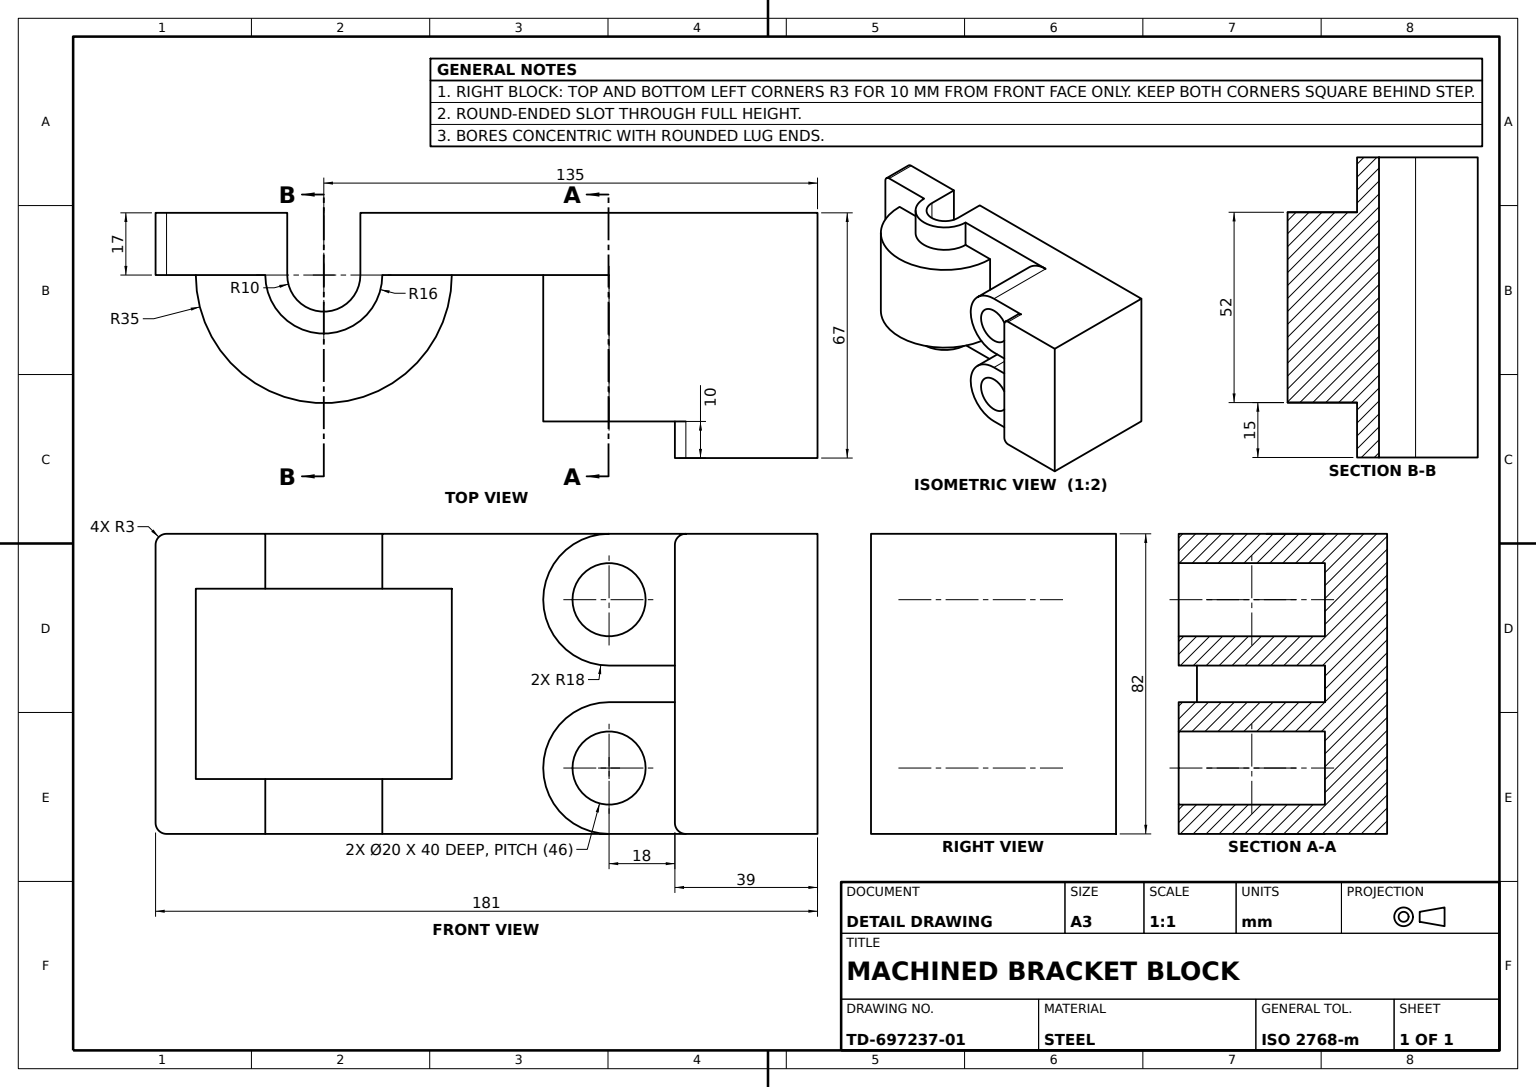
SolidWorks part; units mm, degrees
material "Plain Carbon Steel"
ref_plane "Front Plane" through (0, 0, 0) normal (0, 0, 1) x (1, 0, 0)
ref_plane "Top Plane" through (0, 0, 0) normal (0, 1, 0) x (1, 0, 0)
ref_plane "Right Plane" through (0, 0, 0) normal (1, 0, 0) x (0, 0, -1)
sketch "Base Block Sketch" plane through (0, 0, 0) normal (0, 0, 1) x (1, 0, 0)
  line L3 (0, 0) -> (175, 0)
  line L4 (175, 0) -> (175, 82)
  line L5 (175, 82) -> (0, 82)
  line L6 (0, 82) -> (0, 0)
  dimension "D1" = 175
  dimension "D2" = 82
extrude "Base Block" add sketch "Base Block Sketch" along normal blind 17
sketch "Side Wall Sketch" plane through (0, 0, 17) normal (0, 0, 1) x (1, 0, 0)
  line L0 (175, 82) -> (175, 0)
  line L1 (175, 0) -> (139, 0)
  line L2 (0, 0) -> (175, 0) construction
  line L3 (0, 82) -> (0, 0) construction
  line L4 (175, 82) -> (139, 82)
  line L5 (175, 82) -> (0, 82) construction
  line L7 (136, 79) -> (136, 3)
  arc A0 (136, 3) -> (139, 0) centre (139, 3) ccw
  arc A1 (139, 82) -> (136, 79) centre (139, 79) ccw
  dimension "D1" = 6
  dimension "D2" = 6
  dimension "D3" = 3
  dimension "D4" = 136
extrude "Side Wall" add sketch "Side Wall Sketch" along normal blind 50
sketch "Step Pad Sketch" plane through (0, 0, 0) normal (-1, 0, 0) x (0, 0, 1)
  line L0 (0, 82) -> (17, 82)
  line L1 (17, 82) -> (17, 0)
  line L2 (17, 82) -> (17, 0) construction
  line L3 (17, 0) -> (0, 0) construction
  line L4 (17, 0) -> (0, 0)
  line L5 (0, 82) -> (0, 0)
extrude "Step Pad" add sketch "Step Pad Sketch" along normal blind 3
sketch "Raised Block Sketch" plane through (0, 0, 17) normal (0, 0, 1) x (1, 0, 0)
  line L0 (-3, 82) -> (-3, 0)
  line L1 (-3, 0) -> (-3, 82) construction
  line L3 (-6, 79) -> (-6, 3)
  arc A0 (-3, 82) -> (-6, 79) centre (-3, 79) ccw
  arc A1 (-6, 3) -> (-3, 0) centre (-3, 3) ccw
  dimension "D1" = 3
extrude "Raised Block" add sketch "Raised Block Sketch" against normal blind 17
sketch "Lug Boss Sketch" plane through (0, 0, 0) normal (0, -1, 0) x (1, 0, 0)
  line L0 (175, 0) -> (40, 0)
  line L1 (-3, 0) -> (175, 0) construction
  line L2 (175, 67) -> (175, 0) construction
  line L3 (-3, 17) -> (139, 17) construction
  line L4 (5, 17) -> (75, 17)
  arc A0 (75, 17) -> (5, 17) centre (40, 17) ccw
  line M5 (139, 17) -> (-3, 17)
  dimension "D1" = 35
  dimension "D2" = 135
extrude "Lug Boss" add sketch "Lug Boss Sketch" against normal blind 82 contours A0 M5
sketch "Lug Profile Cut Sketch" plane through (0, 0, 0) normal (0, -1, 0) x (1, 0, 0)
  line L0 (30, 0) -> (50, 0)
  line L1 (30, 17) -> (30, 0)
  line L2 (-3, 0) -> (175, 0) construction
  line L3 (50, 17) -> (50, 0)
  arc A0 (50, 17) -> (30, 17) centre (40, 17) ccw
  dimension "D1" = 10
extrude "Lug Profile Cut" cut sketch "Lug Profile Cut Sketch" against normal blind 82
sketch "Knuckle Slot 1 Sketch" plane through (0, 0, 0) normal (0, -1, 0) x (1, 0, 0)
  line L1 (5, 17) -> (30, 17)
  line L2 (50, 17) -> (75, 17)
  arc A0 (75, 17) -> (5, 17) centre (40, 17) ccw
  arc A1 (50, 17) -> (30, 17) centre (40, 17) ccw
extrude "Knuckle Slot 1" cut sketch "Knuckle Slot 1 Sketch" against normal blind 15
sketch "Knuckle Slot 2 Sketch" plane through (0, 82, 0) normal (0, 1, 0) x (1, 0, 0)
  line L0 (30, -17) -> (5, -17)
  line L1 (50, -17) -> (75, -17)
  arc A0 (5, -17) -> (75, -17) centre (40, -17) ccw
  arc A1 (30, -17) -> (50, -17) centre (40, -17) ccw
extrude "Knuckle Slot 2" cut sketch "Knuckle Slot 2 Sketch" against normal blind 15
sketch "Knuckle Ring 2 Sketch" plane through (0, 67, 0) normal (0, 1, 0) x (1, 0, 0)
  line L0 (24, -17) -> (30, -17)
  line L1 (50, -17) -> (56, -17)
  arc A0 (24, -17) -> (56, -17) centre (40, -17) ccw
  arc A1 (30, -17) -> (50, -17) centre (40, -17) ccw
  dimension "D1" = 16
extrude "Knuckle Ring 2" add sketch "Knuckle Ring 2 Sketch" along normal blind 15
sketch "Knuckle Ring 1 Sketch" plane through (0, 15, 0) normal (0, -1, 0) x (1, 0, 0)
  line L0 (24, 17) -> (30, 17)
  line L1 (50, 17) -> (56, 17)
  arc A0 (56, 17) -> (24, 17) centre (40, 17) ccw
  arc A1 (50, 17) -> (30, 17) centre (40, 17) ccw
  dimension "D1" = 16
  dimension "D2" = 10
extrude "Knuckle Ring 1" add sketch "Knuckle Ring 1 Sketch" along normal blind 15
sketch "Curved Bracket Sketch" plane through (0, 0, 17) normal (0, 0, 1) x (1, 0, 0)
  line L0 (118, 0) -> (139, 0)
  line L1 (118, 82) -> (139, 82)
  line L2 (139, 82) -> (56, 82) construction
  line L3 (118, 46) -> (136, 46)
  line L4 (136, 36) -> (136, 3)
  line L5 (136, 46) -> (136, 79)
  line L6 (136, 79) -> (136, 3) construction
  line L7 (118, 36) -> (136, 36)
  arc A0 (118, 82) -> (118, 46) centre (118, 64) ccw
  arc A1 (118, 36) -> (118, 0) centre (118, 18) ccw
  arc A2 (139, 82) -> (136, 79) centre (139, 79) ccw construction
  arc A3 (136, 3) -> (139, 0) centre (139, 3) ccw
  arc A4 (139, 82) -> (136, 79) centre (139, 79) ccw
  dimension "D1" = 18
extrude "Curved Bracket" add sketch "Curved Bracket Sketch" along normal blind 40
sketch "Bracket Trim Cut Sketch" plane through (0, 0, 57) normal (0, 0, 1) x (1, 0, 0)
  circle A0 centre (118, 64) radius 10
  circle A1 centre (118, 18) radius 10
  dimension "D1" = 20
extrude "Bracket Trim Cut" cut sketch "Bracket Trim Cut Sketch" against normal blind 40
